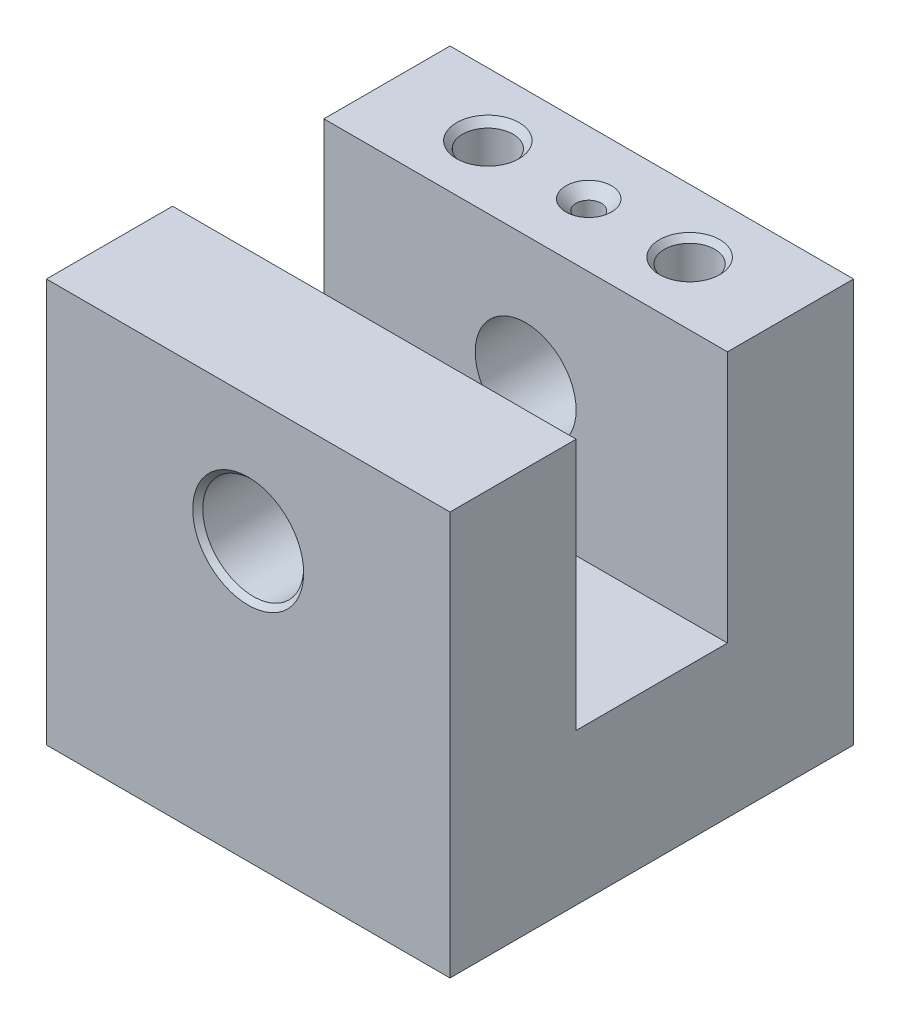
from build123d import *

# Parameters (mm, degrees)
BASE_BLOCK_DEPTH         = 25.4
DOWEL_HOLE_0_126IN_D     = 3.2004
DOWEL_HOLE_0_126IN_DEPTH = 7.62
DOWEL_HOLE_0_126IN_TIP   = 0.961497163
DOWEL_HOLE_CHAMFER_SIZE  = 1.27
BORE_0_5IN_THRU_D        = 12.7
BORE_EDGE_CHAMFER_SIZE   = 0.635


with BuildPart() as part:
    # Base Block Profile Sketch → Base Block (new, symmetric)
    with BuildSketch(Plane(origin=(0, 0, 0), x_dir=(0, 0, -1), z_dir=(1, 0, 0))):
        Polygon((-9.525, 0), (9.525, 0), (9.525, 31.75), (25.4, 31.75), (25.4, 0), (25.4, -19.05), (-25.4, -19.05), (-25.4, 0), (-25.4, 31.75), (-9.525, 31.75), align=None)
    extrude(amount=BASE_BLOCK_DEPTH, both=True)

    # Dowel Hole 0.126in
    with Locations(Plane(origin=(0, 31.75, -17.4625), x_dir=(0, 0, 1), z_dir=(0, 1, 0))):
        with Locations((0, 0)):
            Hole(DOWEL_HOLE_0_126IN_D / 2, depth=DOWEL_HOLE_0_126IN_DEPTH)
            with Locations((0, 0, -(DOWEL_HOLE_0_126IN_DEPTH + DOWEL_HOLE_0_126IN_TIP / 2))):  # 118° drill point
                Cone(0, DOWEL_HOLE_0_126IN_D / 2, DOWEL_HOLE_0_126IN_TIP, mode=Mode.SUBTRACT)

    # Dowel Hole Chamfer
    dowel_hole_chamfer_edges = [part.edges().sort_by_distance(p)[0] for p in [
        (0, 31.75, -15.8623),
    ]]
    chamfer(dowel_hole_chamfer_edges, length=DOWEL_HOLE_CHAMFER_SIZE)

    # Sketch5 → Tapped Hole M-quarter-20 A (revolve, cut)
    with BuildSketch(Plane(origin=(12.7, 31.75, -17.4625), x_dir=(0, 0, 1), z_dir=(1, 0, 0))):
        Polygon((0, 0), (0, 19.0627), (2.5527, 16.51), (2.5527, 12.7), (3.175, 12.7), (3.175, 0.730483939), (3.81, 0), align=None)
    revolve(axis=Axis((12.7, 38.1, -17.4625), (0, -1, 0)), mode=Mode.SUBTRACT)

    # Sketch6 → Tapped Hole M-quarter-20 B (revolve, cut)
    with BuildSketch(Plane(origin=(-12.7, 31.75, -17.4625), x_dir=(0, 0, 1), z_dir=(1, 0, 0))):
        Polygon((0, 0), (0, 19.0627), (2.5527, 16.51), (2.5527, 12.7), (3.175, 12.7), (3.175, 0.876580726), (3.937, 0), align=None)
    revolve(axis=Axis((-12.7, 38.1, -17.4625), (0, -1, 0)), mode=Mode.SUBTRACT)

    # Bore 0.5in Thru (through all)
    with Locations(Plane(origin=(0, 15.875, 25.4), x_dir=(0, 1, 0), z_dir=(0, 0, 1))):
        with Locations((0, 0)):
            Hole(BORE_0_5IN_THRU_D / 2)

    # Bore Edge Chamfer
    bore_edge_chamfer_edges = [part.edges().sort_by_distance(p)[0] for p in [
        (0, 22.225, -25.4),
        (0, 22.225, 25.4),
    ]]
    chamfer(bore_edge_chamfer_edges, length=BORE_EDGE_CHAMFER_SIZE)


solid = part.part
